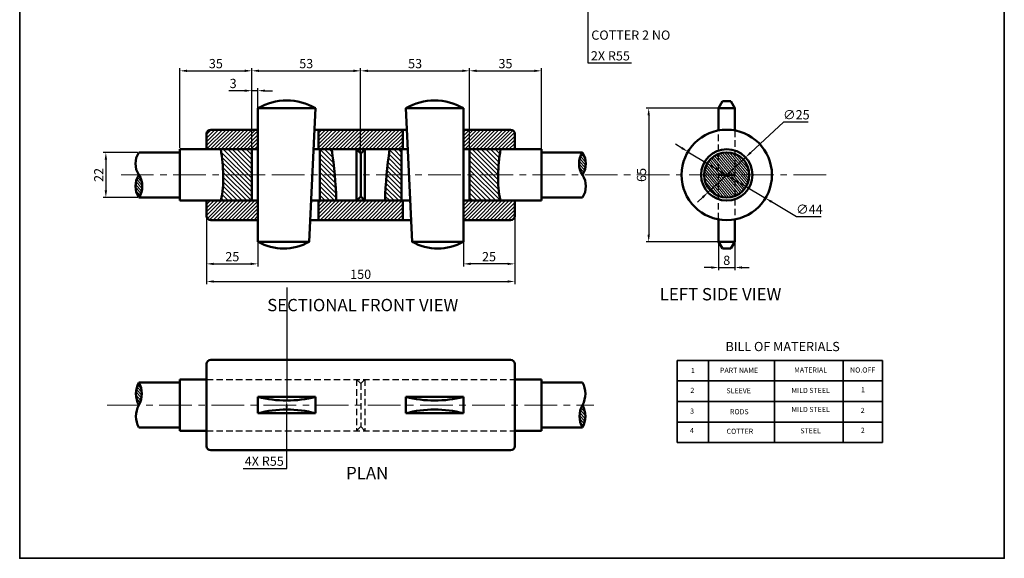
# Model space of a CAD drawing. Units: millimetres. Extents: x -431 to 49, y 153 to 670.
# Tile 1 of 2: x -431 to 49, y 153 to 415. Entities that reach past the tile are written whole.
import ezdxf

# ---------------------------------------------------------------- set-up
doc = ezdxf.new("R2010")
doc.units = ezdxf.units.MM
doc.header["$LTSCALE"] = 0.5
doc.linetypes.add('CENTER', pattern=[50.8, 31.75, -6.35, 6.35, -6.35])
doc.linetypes.add('HIDDEN', pattern=[9.525, 6.35, -3.175])
for name, color, linetype, lineweight in [('M-CNTR', 1, 'CENTER', 18), ('M-DIMS', 2, 'Continuous', 25), ('M-HATC', 8, 'Continuous', 18), ('M-HIDN', 6, 'HIDDEN', 25), ('M-OUTL', 7, 'Continuous', 50), ('M-TEXT', 3, 'Continuous', 25), ('M-TTLB', 7, 'Continuous', 35)]:
    doc.layers.add(name, color=color, linetype=linetype, lineweight=lineweight)
doc.styles.get("Standard").update_dxf_attribs({"font": 'arial.ttf'})
doc.dimstyles.new('ISO-25', dxfattribs={"dimtxt": 4.5, "dimasz": 3.5, "dimexe": 1.25, "dimexo": 0.625, "dimtad": 1, "dimtoh": 1, "dimdec": 0, "dimtxsty": 'Standard', "dimcen": 2.5, "dimadec": 0, "dimazin": 0, "dimtfac": 1, "dimtdec": 0, "dimtmove": 0, "dimatfit": 3, "dimfxl": 1, "dimarcsym": 0})

# ---------------------------------------------------------------- blocks, each defined once
blk = doc.blocks.new('*D14')
at = {"layer": 'Defpoints', "color": 0, "transparency": 16777216}
for p in [(-372.61, 350.31), (-388.68, 328.31), (-372.61, 328.31)]:
    blk.add_point(p, dxfattribs=at)
at = {"layer": 'M-DIMS', "color": 0, "lineweight": -2, "transparency": 16777216}
for p, q in [((-373.23, 350.31), (-389.93, 350.31)), ((-388.68, 346.81), (-388.68, 331.81)), ((-373.23, 328.31), (-389.93, 328.31))]:
    blk.add_line(p, q, dxfattribs=at)
at = {"layer": 'M-DIMS', "color": 0, "transparency": 16777216}
for points in [[(-389.26, 346.81), (-388.1, 346.81), (-388.68, 350.31)], [(-389.26, 331.81), (-388.1, 331.81), (-388.68, 328.31)]]:
    blk.add_solid(points, dxfattribs=at)
at = {"layer": 'M-DIMS', "color": 0, "transparency": 16777216, "insert": (-391.56, 339.31), "char_height": 4.5, "attachment_point": 5, "rotation": 90}
blk.add_mtext('22', dxfattribs=at)
blk = doc.blocks.new('*D15')
at = {"layer": 'Defpoints', "color": 0, "transparency": 16777216}
for p in [(-317.61, 389.99), (-352.61, 351.81), (-317.61, 351.81)]:
    blk.add_point(p, dxfattribs=at)
at = {"layer": 'M-DIMS', "color": 0, "lineweight": -2, "transparency": 16777216}
for p, q in [((-352.61, 352.44), (-352.61, 391.24)), ((-349.11, 389.99), (-321.11, 389.99)), ((-317.61, 352.44), (-317.61, 391.24))]:
    blk.add_line(p, q, dxfattribs=at)
at = {"layer": 'M-DIMS', "color": 0, "transparency": 16777216}
for points in [[(-349.11, 390.58), (-349.11, 389.41), (-352.61, 389.99)], [(-321.11, 390.58), (-321.11, 389.41), (-317.61, 389.99)]]:
    blk.add_solid(points, dxfattribs=at)
at = {"layer": 'M-DIMS', "color": 0, "transparency": 16777216, "insert": (-335.11, 392.92), "char_height": 4.5, "attachment_point": 5}
blk.add_mtext('35', dxfattribs=at)
blk = doc.blocks.new('*D16')
at = {"layer": 'Defpoints', "color": 0, "transparency": 16777216}
for p in [(-317.61, 380.32), (-317.61, 351.81), (-314.61, 351.81)]:
    blk.add_point(p, dxfattribs=at)
at = {"layer": 'M-DIMS', "color": 0, "lineweight": -2, "transparency": 16777216}
for p, q in [((-321.11, 380.32), (-328.81, 380.32)), ((-317.61, 352.44), (-317.61, 381.57)), ((-314.61, 380.32), (-317.61, 380.32)), ((-314.61, 352.44), (-314.61, 381.57)), ((-311.11, 380.32), (-307.61, 380.32))]:
    blk.add_line(p, q, dxfattribs=at)
at = {"layer": 'M-DIMS', "color": 0, "transparency": 16777216}
for points in [[(-321.11, 380.9), (-321.11, 379.74), (-317.61, 380.32)], [(-311.11, 380.9), (-311.11, 379.74), (-314.61, 380.32)]]:
    blk.add_solid(points, dxfattribs=at)
at = {"layer": 'M-DIMS', "color": 0, "transparency": 16777216, "insert": (-326.71, 383.25), "char_height": 4.5, "attachment_point": 5}
blk.add_mtext('3', dxfattribs=at)
blk = doc.blocks.new('*D17')
at = {"layer": 'Defpoints', "color": 0, "transparency": 16777216}
for p in [(-264.61, 389.99), (-317.61, 339.31), (-264.61, 339.31)]:
    blk.add_point(p, dxfattribs=at)
at = {"layer": 'M-DIMS', "color": 0, "lineweight": -2, "transparency": 16777216}
for p, q in [((-317.61, 339.94), (-317.61, 391.24)), ((-314.11, 389.99), (-268.11, 389.99)), ((-264.61, 339.94), (-264.61, 391.24))]:
    blk.add_line(p, q, dxfattribs=at)
at = {"layer": 'M-DIMS', "color": 0, "transparency": 16777216}
for points in [[(-314.11, 390.58), (-314.11, 389.41), (-317.61, 389.99)], [(-268.11, 390.58), (-268.11, 389.41), (-264.61, 389.99)]]:
    blk.add_solid(points, dxfattribs=at)
at = {"layer": 'M-DIMS', "color": 0, "transparency": 16777216, "insert": (-291.11, 392.92), "char_height": 4.5, "attachment_point": 5}
blk.add_mtext('53', dxfattribs=at)
blk = doc.blocks.new('*D18')
at = {"layer": 'Defpoints', "color": 0, "transparency": 16777216}
for p in [(-211.61, 389.99), (-264.61, 339.31), (-211.61, 339.31)]:
    blk.add_point(p, dxfattribs=at)
at = {"layer": 'M-DIMS', "color": 0, "lineweight": -2, "transparency": 16777216}
for p, q in [((-264.61, 339.94), (-264.61, 391.24)), ((-261.11, 389.99), (-215.11, 389.99)), ((-211.61, 339.94), (-211.61, 391.24))]:
    blk.add_line(p, q, dxfattribs=at)
at = {"layer": 'M-DIMS', "color": 0, "transparency": 16777216}
for points in [[(-261.11, 390.58), (-261.11, 389.41), (-264.61, 389.99)], [(-215.11, 390.58), (-215.11, 389.41), (-211.61, 389.99)]]:
    blk.add_solid(points, dxfattribs=at)
at = {"layer": 'M-DIMS', "color": 0, "transparency": 16777216, "insert": (-238.11, 392.92), "char_height": 4.5, "attachment_point": 5}
blk.add_mtext('53', dxfattribs=at)
blk = doc.blocks.new('*D19')
at = {"layer": 'Defpoints', "color": 0, "transparency": 16777216}
for p in [(-176.61, 389.99), (-211.61, 339.31), (-176.61, 339.31)]:
    blk.add_point(p, dxfattribs=at)
at = {"layer": 'M-DIMS', "color": 0, "lineweight": -2, "transparency": 16777216}
for p, q in [((-211.61, 339.94), (-211.61, 391.24)), ((-208.11, 389.99), (-180.11, 389.99)), ((-176.61, 339.94), (-176.61, 391.24))]:
    blk.add_line(p, q, dxfattribs=at)
at = {"layer": 'M-DIMS', "color": 0, "transparency": 16777216}
for points in [[(-208.11, 390.58), (-208.11, 389.41), (-211.61, 389.99)], [(-180.11, 390.58), (-180.11, 389.41), (-176.61, 389.99)]]:
    blk.add_solid(points, dxfattribs=at)
at = {"layer": 'M-DIMS', "color": 0, "transparency": 16777216, "insert": (-194.11, 392.92), "char_height": 4.5, "attachment_point": 5}
blk.add_mtext('35', dxfattribs=at)
blk = doc.blocks.new('*D20')
at = {"layer": 'Defpoints', "color": 0, "transparency": 16777216}
for p in [(-189.61, 326.81), (-339.61, 319.31), (-189.61, 287.45)]:
    blk.add_point(p, dxfattribs=at)
at = {"layer": 'M-DIMS', "color": 0, "lineweight": -2, "transparency": 16777216}
for p, q in [((-189.61, 326.19), (-189.61, 286.2)), ((-339.61, 318.69), (-339.61, 286.2)), ((-336.11, 287.45), (-193.11, 287.45))]:
    blk.add_line(p, q, dxfattribs=at)
at = {"layer": 'M-DIMS', "color": 0, "transparency": 16777216}
for points in [[(-336.11, 288.03), (-336.11, 286.87), (-339.61, 287.45)], [(-193.11, 288.03), (-193.11, 286.87), (-189.61, 287.45)]]:
    blk.add_solid(points, dxfattribs=at)
at = {"layer": 'M-DIMS', "color": 0, "transparency": 16777216, "insert": (-264.61, 290.37), "char_height": 4.5, "attachment_point": 5}
blk.add_mtext('150', dxfattribs=at)
blk = doc.blocks.new('*D21')
at = {"layer": 'Defpoints', "color": 0, "transparency": 16777216}
for p in [(-339.61, 321.31), (-314.61, 321.31), (-314.61, 296.03)]:
    blk.add_point(p, dxfattribs=at)
at = {"layer": 'M-DIMS', "color": 0, "lineweight": -2, "transparency": 16777216}
for p, q in [((-339.61, 320.69), (-339.61, 294.78)), ((-314.61, 320.69), (-314.61, 294.78)), ((-336.11, 296.03), (-318.11, 296.03))]:
    blk.add_line(p, q, dxfattribs=at)
at = {"layer": 'M-DIMS', "color": 0, "transparency": 16777216}
for points in [[(-336.11, 296.61), (-336.11, 295.45), (-339.61, 296.03)], [(-318.11, 296.61), (-318.11, 295.45), (-314.61, 296.03)]]:
    blk.add_solid(points, dxfattribs=at)
at = {"layer": 'M-DIMS', "color": 0, "transparency": 16777216, "insert": (-327.11, 298.95), "char_height": 4.5, "attachment_point": 5}
blk.add_mtext('25', dxfattribs=at)
blk = doc.blocks.new('*D22')
at = {"layer": 'Defpoints', "color": 0, "transparency": 16777216}
for p in [(-214.61, 323.06), (-189.61, 323.06), (-214.61, 296.03)]:
    blk.add_point(p, dxfattribs=at)
at = {"layer": 'M-DIMS', "color": 0, "lineweight": -2, "transparency": 16777216}
for p, q in [((-214.61, 322.44), (-214.61, 294.78)), ((-189.61, 322.44), (-189.61, 294.78)), ((-193.11, 296.03), (-211.11, 296.03))]:
    blk.add_line(p, q, dxfattribs=at)
at = {"layer": 'M-DIMS', "color": 0, "transparency": 16777216}
for points in [[(-211.11, 296.61), (-211.11, 295.45), (-214.61, 296.03)], [(-193.11, 296.61), (-193.11, 295.45), (-189.61, 296.03)]]:
    blk.add_solid(points, dxfattribs=at)
at = {"layer": 'M-DIMS', "color": 0, "transparency": 16777216, "insert": (-202.11, 298.95), "char_height": 4.5, "attachment_point": 5}
blk.add_mtext('25', dxfattribs=at)
blk = doc.blocks.new('*D23')
at = {"layer": 'Defpoints', "color": 0, "transparency": 16777216}
for p in [(-105.24, 350.62), (-67.5, 328.01)]:
    blk.add_point(p, dxfattribs=at)
at = {"layer": 'M-DIMS', "color": 0, "lineweight": -2, "transparency": 16777216}
for p, q in [((-108.24, 352.42), (-111.24, 354.22)), ((-105.24, 350.62), (-67.5, 328.01)), ((-52.4, 318.96), (-64.49, 326.21)), ((-40.45, 318.96), (-52.4, 318.96))]:
    blk.add_line(p, q, dxfattribs=at)
at = {"layer": 'M-DIMS', "color": 0, "transparency": 16777216}
for points in [[(-107.94, 352.92), (-108.54, 351.92), (-105.24, 350.62)], [(-64.19, 326.71), (-64.79, 325.71), (-67.5, 328.01)]]:
    blk.add_solid(points, dxfattribs=at)
at = {"layer": 'M-DIMS', "color": 0, "transparency": 16777216, "insert": (-46.12, 322.01), "char_height": 4.5, "attachment_point": 5}
blk.add_mtext('∅44', dxfattribs=at)
blk = doc.blocks.new('*D24')
at = {"layer": 'Defpoints', "color": 0, "transparency": 16777216}
for p in [(-77.22, 347.83), (-95.52, 330.8)]:
    blk.add_point(p, dxfattribs=at)
at = {"layer": 'M-DIMS', "color": 0, "lineweight": -2, "transparency": 16777216}
for p, q in [((-58.78, 364.97), (-74.65, 350.21)), ((-46.78, 364.97), (-58.78, 364.97)), ((-95.52, 330.8), (-77.22, 347.83)), ((-98.08, 328.42), (-100.65, 326.03))]:
    blk.add_line(p, q, dxfattribs=at)
at = {"layer": 'M-DIMS', "color": 0, "transparency": 16777216}
for points in [[(-75.05, 350.64), (-74.26, 349.78), (-77.22, 347.83)], [(-98.48, 328.84), (-97.69, 327.99), (-95.52, 330.8)]]:
    blk.add_solid(points, dxfattribs=at)
at = {"layer": 'M-DIMS', "color": 0, "transparency": 16777216, "insert": (-52.47, 368.02), "char_height": 4.5, "attachment_point": 5}
blk.add_mtext('∅25', dxfattribs=at)
blk = doc.blocks.new('*D25')
at = {"layer": 'Defpoints', "color": 0, "transparency": 16777216}
for p in [(-90.37, 306.81), (-82.37, 306.81), (-82.37, 294.26)]:
    blk.add_point(p, dxfattribs=at)
at = {"layer": 'M-DIMS', "color": 0, "lineweight": -2, "transparency": 16777216}
for p, q in [((-90.37, 306.19), (-90.37, 293.01)), ((-82.37, 306.19), (-82.37, 293.01)), ((-93.87, 294.26), (-97.37, 294.26)), ((-90.37, 294.26), (-82.37, 294.26)), ((-78.87, 294.26), (-75.37, 294.26))]:
    blk.add_line(p, q, dxfattribs=at)
at = {"layer": 'M-DIMS', "color": 0, "transparency": 16777216}
for points in [[(-93.87, 294.84), (-93.87, 293.67), (-90.37, 294.26)], [(-78.87, 294.84), (-78.87, 293.67), (-82.37, 294.26)]]:
    blk.add_solid(points, dxfattribs=at)
at = {"layer": 'M-DIMS', "color": 0, "transparency": 16777216, "insert": (-86.37, 297.18), "char_height": 4.5, "attachment_point": 5}
blk.add_mtext('8', dxfattribs=at)
blk = doc.blocks.new('*D26')
at = {"layer": 'Defpoints', "color": 0, "transparency": 16777216}
for p in [(-86.37, 371.81), (-124.36, 306.81), (-86.37, 306.81)]:
    blk.add_point(p, dxfattribs=at)
at = {"layer": 'M-DIMS', "color": 0, "lineweight": -2, "transparency": 16777216}
for p, q in [((-86.99, 371.81), (-125.61, 371.81)), ((-124.36, 368.31), (-124.36, 310.31)), ((-86.99, 306.81), (-125.61, 306.81))]:
    blk.add_line(p, q, dxfattribs=at)
at = {"layer": 'M-DIMS', "color": 0, "transparency": 16777216}
for points in [[(-124.95, 368.31), (-123.78, 368.31), (-124.36, 371.81)], [(-124.95, 310.31), (-123.78, 310.31), (-124.36, 306.81)]]:
    blk.add_solid(points, dxfattribs=at)
at = {"layer": 'M-DIMS', "color": 0, "transparency": 16777216, "insert": (-127.29, 339.31), "char_height": 4.5, "attachment_point": 5, "rotation": 90}
blk.add_mtext('65', dxfattribs=at)
blk = doc.blocks.new('COTTER-FRONT')
blk.add_lwpolyline([(28, 65), (28, 0), (3, 0), (0, 65)], close=True)
blk.add_arc((14, 40.75), 28, 60, 120)
blk = doc.blocks.new('COTTER-TOP')
for p, q in [((28, 8), (0, 8)), ((0, 8), (0, 0)), ((28, 0), (28, 8)), ((0, 0), (28, 0))]:
    blk.add_line(p, q)
for centre, start, end in [((14, 61.19), 255.2533, 284.7467), ((14, -53.19), 75.2533, 104.7467)]:
    blk.add_arc(centre, 55, start, end)
blk = doc.blocks.new('*D34')
at = {"layer": 'Defpoints', "color": 0, "ltscale": 0.5, "transparency": 16777216}
for p in [(-153.92, 481.78), (-153.91, 426.78)]:
    blk.add_point(p, dxfattribs=at)
at = {"layer": 'M-DIMS', "color": 0, "lineweight": -2, "ltscale": 0.5, "transparency": 16777216}
for p, q in [((-153.92, 481.78), (-153.91, 426.78)), ((-153.91, 393.78), (-153.91, 423.28)), ((-132.76, 393.78), (-153.91, 393.78))]:
    blk.add_line(p, q, dxfattribs=at)
at = {"layer": 'M-DIMS', "color": 0, "ltscale": 0.5, "transparency": 16777216}
blk.add_solid([(-153.33, 423.28), (-154.5, 423.28), (-153.91, 426.78)], dxfattribs=at)
at = {"layer": 'M-DIMS', "color": 0, "ltscale": 0.5, "transparency": 16777216, "insert": (-143.02, 396.71), "char_height": 4.5, "attachment_point": 5}
blk.add_mtext('2X R55', dxfattribs=at)
blk = doc.blocks.new('*D35')
at = {"layer": 'Defpoints', "color": 0, "ltscale": 0.5, "transparency": 16777216}
for p in [(-300.61, 284.5), (-300.61, 229.5)]:
    blk.add_point(p, dxfattribs=at)
at = {"layer": 'M-DIMS', "color": 0, "lineweight": -2, "ltscale": 0.5, "transparency": 16777216}
for p, q in [((-300.61, 284.5), (-300.61, 229.5)), ((-300.61, 196.5), (-300.61, 226)), ((-321.87, 196.5), (-300.61, 196.5))]:
    blk.add_line(p, q, dxfattribs=at)
at = {"layer": 'M-DIMS', "color": 0, "ltscale": 0.5, "transparency": 16777216}
blk.add_solid([(-301.19, 226), (-300.03, 226), (-300.61, 229.5)], dxfattribs=at)
at = {"layer": 'M-DIMS', "color": 0, "ltscale": 0.5, "transparency": 16777216, "insert": (-311.55, 199.41), "char_height": 4.5, "attachment_point": 5}
blk.add_mtext('4X R55', dxfattribs=at)

msp = doc.modelspace()

# ---------------------------------------------------------------- hatches: boundary and pattern name
at = {"layer": 'M-HATC'}
h = msp.add_hatch(dxfattribs=at)
h.set_pattern_fill('ANSI31', color=256, scale=0.4)
h.paths.add_polyline_path([(-314.609, 361.3128), (-337.609, 361.3128, 0.41421356), (-339.609, 359.3128), (-339.609, 351.8128), (-314.609, 351.8128)])
h.paths.add_polyline_path([(-244.1244, 361.3128), (-285.0936, 361.3128), (-285.0936, 351.8128), (-244.1244, 351.8128)])
h.paths.add_polyline_path([(-189.609, 359.3128, 0.41421356), (-191.609, 361.3128), (-214.609, 361.3128), (-214.609, 351.8128), (-189.609, 351.8128)])
h.paths.add_polyline_path([(-189.609, 326.8128), (-214.609, 326.8128), (-214.609, 317.3128), (-191.609, 317.3128, 0.41421356), (-189.609, 319.3128)])
h.paths.add_polyline_path([(-244.1244, 326.8128), (-285.0936, 326.8128), (-285.0936, 317.3128), (-244.1244, 317.3128)])
h.paths.add_polyline_path([(-314.609, 326.8128), (-339.609, 326.8128), (-339.609, 319.3128, 0.41421356), (-337.609, 317.3128), (-314.609, 317.3128)])
h = msp.add_hatch(dxfattribs=at)
h.set_pattern_fill('ANSI31', color=256, scale=0.5, angle=90)
edge = h.paths.add_edge_path()
edge.add_line((-317.609, 351.8128), (-332.6455, 351.8128))
edge.add_spline(control_points=[(-332.6455, 351.8128), (-332.1521, 347.6251), (-331.6587, 343.4374), (-331.5237, 339.3128)], knot_values=[0, 0, 0, 0, 12.30275825, 12.30275825, 12.30275825, 12.30275825], degree=3, periodic=0)
edge.add_line((-331.5237, 339.3128), (-317.609, 339.3128))
edge.add_line((-317.609, 339.3128), (-317.609, 351.8128))
edge = h.paths.add_edge_path()
edge.add_line((-317.609, 339.3128), (-331.5237, 339.3128))
edge.add_spline(control_points=[(-331.5237, 339.3128), (-331.3844, 335.0558), (-331.627, 330.8661), (-332.6455, 326.8128)], knot_values=[12.30275825, 12.30275825, 12.30275825, 12.30275825, 25, 25, 25, 25], degree=3, periodic=0)
edge.add_line((-332.6455, 326.8128), (-317.609, 326.8128))
edge.add_line((-317.609, 326.8128), (-317.609, 339.3128))
edge = h.paths.add_edge_path()
edge.add_spline(control_points=[(-277.2476, 339.3128), (-277.6434, 343.4827), (-278.1538, 347.6477), (-278.6643, 351.8128)], knot_values=[0, 0, 0, 0, 12.56066367, 12.56066367, 12.56066367, 12.56066367], degree=3, periodic=0)
edge.add_line((-278.6643, 351.8128), (-284.5321, 351.8128))
edge.add_line((-284.5321, 351.8128), (-284.5321, 339.3128))
edge.add_line((-284.5321, 339.3128), (-277.2476, 339.3128))
edge = h.paths.add_edge_path()
edge.add_spline(control_points=[(-276.5193, 326.8128), (-276.572, 330.9876), (-276.8527, 335.1526), (-277.2476, 339.3128)], knot_values=[12.56066367, 12.56066367, 12.56066367, 12.56066367, 25.09185019, 25.09185019, 25.09185019, 25.09185019], degree=3, periodic=0)
edge.add_line((-277.2476, 339.3128), (-284.5321, 339.3128))
edge.add_line((-284.5321, 339.3128), (-284.5321, 326.8128))
edge.add_line((-284.5321, 326.8128), (-276.5193, 326.8128))
h = msp.add_hatch(dxfattribs=at)
h.set_pattern_fill('ANSI31', color=256, scale=0.5, angle=90)
edge = h.paths.add_edge_path()
edge.add_line((-211.609, 351.8128), (-196.5725, 351.8128))
edge.add_spline(control_points=[(-196.5725, 351.8128), (-197.0659, 347.6251), (-197.5594, 343.4374), (-197.6943, 339.3128)], knot_values=[0, 0, 0, 0, 12.30275825, 12.30275825, 12.30275825, 12.30275825], degree=3, periodic=0)
edge.add_line((-197.6943, 339.3128), (-211.609, 339.3128))
edge.add_line((-211.609, 339.3128), (-211.609, 351.8128))
edge = h.paths.add_edge_path()
edge.add_line((-211.609, 339.3128), (-197.6943, 339.3128))
edge.add_spline(control_points=[(-197.6943, 339.3128), (-197.8336, 335.0558), (-197.591, 330.8661), (-196.5725, 326.8128)], knot_values=[12.30275825, 12.30275825, 12.30275825, 12.30275825, 25, 25, 25, 25], degree=3, periodic=0)
edge.add_line((-196.5725, 326.8128), (-211.609, 326.8128))
edge.add_line((-211.609, 326.8128), (-211.609, 339.3128))
edge = h.paths.add_edge_path()
edge.add_spline(control_points=[(-251.9704, 339.3128), (-251.5746, 343.4827), (-251.0642, 347.6477), (-250.5537, 351.8128)], knot_values=[0, 0, 0, 0, 12.56066367, 12.56066367, 12.56066367, 12.56066367], degree=3, periodic=0)
edge.add_line((-250.5537, 351.8128), (-244.6859, 351.8128))
edge.add_line((-244.6859, 351.8128), (-244.6859, 339.3128))
edge.add_line((-244.6859, 339.3128), (-251.9704, 339.3128))
edge = h.paths.add_edge_path()
edge.add_spline(control_points=[(-252.6987, 326.8128), (-252.646, 330.9876), (-252.3653, 335.1526), (-251.9704, 339.3128)], knot_values=[12.56066367, 12.56066367, 12.56066367, 12.56066367, 25.09185019, 25.09185019, 25.09185019, 25.09185019], degree=3, periodic=0)
edge.add_line((-251.9704, 339.3128), (-244.6859, 339.3128))
edge.add_line((-244.6859, 339.3128), (-244.6859, 326.8128))
edge.add_line((-244.6859, 326.8128), (-252.6987, 326.8128))
h = msp.add_hatch(dxfattribs=at)
h.set_pattern_fill('ANSI31', color=256, scale=0.3, angle=85)
h.set_pattern_definition([(130, (180.36415, 264.273), (-0.7296573, -0.6122552), [])])
h.paths.add_polyline_path([(-156.609, 339.3128, 0.29970063), (-156.609, 350.3128, 0.29970063)])
h = msp.add_hatch(dxfattribs=at)
h.set_pattern_fill('ANSI31', color=256, scale=0.3, angle=85)
h.paths.add_polyline_path([(-90.3682, 349.5597, 0.30896041), (-97.3682, 339.3128), (-90.3682, 339.3128)])
h.paths.add_polyline_path([(-82.3682, 349.5597, 0.18826231), (-90.3682, 349.5597), (-90.3682, 339.3128), (-82.3682, 339.3128)])
h.paths.add_polyline_path([(-82.3682, 339.3128), (-90.3682, 339.3128), (-90.3682, 329.0658, 0.18826231), (-82.3682, 329.0658)])
h.paths.add_polyline_path([(-90.3682, 339.3128), (-97.3682, 339.3128, 0.30896041), (-90.3682, 329.0658)])
h.paths.add_polyline_path([(-82.3682, 349.5597), (-82.3682, 339.3128), (-75.3682, 339.3128, 0.30896041)])
h.paths.add_polyline_path([(-75.3682, 339.3128), (-82.3682, 339.3128), (-82.3682, 329.0658, 0.30896041)])
h = msp.add_hatch(dxfattribs=at)
h.set_pattern_fill('ANSI31', color=256, scale=0.3, angle=85)
h.set_pattern_definition([(130, (-476.5793, 264.273), (-0.729657, -0.612255), [])])
h.paths.add_polyline_path([(-372.609, 339.3128, 0.29970063), (-372.609, 328.3128, 0.29970063)])
h = msp.add_hatch(dxfattribs=at)
h.set_pattern_fill('ANSI31', color=256, scale=0.3, angle=85)
h.paths.add_polyline_path([(-372.609, 238.3094, 0.25704732), (-372.609, 227.3094, 0.25704732)])
h.paths.add_polyline_path([(-156.609, 227.3094, 0.25704732), (-156.609, 216.3094, 0.25704732)])

# ---------------------------------------------------------------- linework, layer by layer
at = {"layer": 'M-CNTR'}
for p, q in [((-314.609, 339.3128), (-383.9378, 339.3128)), ((-38.0264, 339.3128), (-314.609, 339.3128)), ((-388.0686, 227.3094), (-151.045, 227.3094))]:
    msp.add_line(p, q, dxfattribs=at)
at = {"layer": 'M-HIDN'}
for p, q in [((-90.3682, 317.6794), (-90.3682, 360.9461)), ((-82.3682, 360.9461), (-82.3682, 317.6794)), ((-339.609, 239.8094), (-189.609, 239.8094)), ((-266.609, 239.8094), (-264.609, 237.8094)), ((-266.609, 239.8094), (-266.609, 214.8094)), ((-262.609, 239.8094), (-264.609, 237.8094)), ((-262.609, 239.8094), (-262.609, 214.8094)), ((-264.609, 237.8094), (-264.609, 216.8094)), ((-266.609, 214.8094), (-264.609, 216.8094)), ((-262.609, 214.8094), (-264.609, 216.8094)), ((-339.609, 214.8094), (-189.609, 214.8094))]:
    msp.add_line(p, q, dxfattribs=at)
at = {"layer": 'M-OUTL'}
for p, q in [((-88.3682, 375.1621), (-90.3682, 371.8128)), ((-88.3682, 375.1621), (-84.3682, 375.1621)), ((-84.3682, 375.1621), (-82.3682, 371.8128)), ((-90.3682, 371.8128), (-90.3682, 360.9461)), ((-82.3682, 371.8128), (-90.3682, 371.8128)), ((-82.3682, 360.9461), (-82.3682, 371.8128)), ((-314.609, 361.3128), (-337.609, 361.3128)), ((-314.609, 361.3128), (-314.609, 351.8128)), ((-242.1244, 361.3128), (-287.0936, 361.3128)), ((-285.0936, 361.3128), (-285.0936, 351.8128)), ((-242.1244, 361.3128), (-244.1244, 361.3128)), ((-244.1244, 361.3128), (-244.1244, 351.8128)), ((-214.609, 351.8128), (-214.609, 361.3128)), ((-191.609, 361.3128), (-214.609, 361.3128)), ((-339.609, 359.3128), (-339.609, 351.8128)), ((-189.609, 351.8128), (-189.609, 359.3128)), ((-352.609, 350.3128), (-372.609, 350.3128)), ((-352.609, 351.8128), (-314.609, 351.8128)), ((-352.609, 326.8128), (-352.609, 351.8128)), ((-339.609, 351.8128), (-314.609, 351.8128)), ((-317.609, 326.8128), (-317.609, 351.8128)), ((-287.5321, 351.8128), (-266.609, 351.8128)), ((-287.5321, 351.8128), (-241.6859, 351.8128)), ((-284.5321, 351.8128), (-284.5321, 326.8128)), ((-266.609, 351.8128), (-264.609, 349.8128)), ((-266.609, 351.8128), (-266.609, 326.8128)), ((-262.609, 351.8128), (-264.609, 349.8128)), ((-262.609, 351.8128), (-262.609, 326.8128)), ((-241.6859, 351.8128), (-262.609, 351.8128)), ((-244.6859, 351.8128), (-244.6859, 326.8128)), ((-176.609, 351.8128), (-214.609, 351.8128)), ((-214.609, 351.8128), (-189.609, 351.8128)), ((-211.609, 326.8128), (-211.609, 351.8128)), ((-176.609, 326.8128), (-176.609, 351.8128)), ((-176.609, 350.3128), (-156.609, 350.3128)), ((-264.609, 349.8128), (-264.609, 328.8128)), ((-264.609, 349.8128), (-264.609, 328.8128)), ((-82.3682, 339.3128), (-90.3682, 339.3128)), ((-372.609, 328.3128), (-352.609, 328.3128)), ((-314.609, 326.8128), (-352.609, 326.8128)), ((-339.609, 326.8128), (-314.609, 326.8128)), ((-339.609, 326.8128), (-339.609, 319.3128)), ((-314.609, 326.8128), (-314.609, 317.3128)), ((-266.609, 326.8128), (-288.6859, 326.8128)), ((-288.6859, 326.8128), (-240.5321, 326.8128)), ((-285.0936, 326.8128), (-285.0936, 317.3128)), ((-266.609, 326.8128), (-264.609, 328.8128)), ((-262.609, 326.8128), (-264.609, 328.8128)), ((-262.609, 326.8128), (-240.5321, 326.8128)), ((-244.1244, 326.8128), (-244.1244, 317.3128)), ((-214.609, 317.3128), (-214.609, 326.8128)), ((-214.609, 326.8128), (-176.609, 326.8128)), ((-214.609, 326.8128), (-189.609, 326.8128)), ((-189.609, 319.3128), (-189.609, 326.8128)), ((-156.609, 328.3128), (-176.609, 328.3128)), ((-337.609, 317.3128), (-314.609, 317.3128)), ((-289.1244, 317.3128), (-240.0936, 317.3128)), ((-214.609, 317.3128), (-191.609, 317.3128)), ((-90.3682, 317.6794), (-90.3682, 306.8128)), ((-82.3682, 306.8128), (-82.3682, 317.6794)), ((-90.3682, 306.8128), (-82.3682, 306.8128)), ((-88.3682, 303.4634), (-90.3682, 306.8128)), ((-88.3682, 303.4634), (-84.3682, 303.4634)), ((-84.3682, 303.4634), (-82.3682, 306.8128)), ((-191.609, 249.3094), (-337.609, 249.3094)), ((-242.1244, 249.3094), (-244.1244, 249.3094)), ((-339.609, 247.3094), (-339.609, 207.3094)), ((-189.609, 207.3094), (-189.609, 247.3094)), ((-339.609, 239.8094), (-352.609, 239.8094)), ((-352.609, 239.8094), (-352.609, 214.8094)), ((-189.609, 239.8094), (-176.609, 239.8094)), ((-176.609, 239.8094), (-176.609, 214.8094)), ((-352.609, 238.3094), (-372.609, 238.3094)), ((-176.609, 238.3094), (-156.609, 238.3094)), ((-352.609, 216.3094), (-372.609, 216.3094)), ((-176.609, 216.3094), (-156.609, 216.3094)), ((-352.609, 214.8094), (-339.609, 214.8094)), ((-189.609, 214.8094), (-176.609, 214.8094)), ((-337.609, 205.3094), (-191.609, 205.3094))]:
    msp.add_line(p, q, dxfattribs=at)
for radius in [22, 12.5, 11]:
    msp.add_circle((-86.3682, 339.3128), radius, dxfattribs=at)
for centre, radius, start, end in [((-337.609, 359.3128), 2, 90, 180), ((-191.609, 359.3128), 2, 0, 90), ((-364.2574, 344.8128), 10, 146.632987, 213.367013), ((-148.2574, 344.8128), 10, 146.632987, 213.367013), ((-164.9607, 344.8128), 10, 326.632987, 33.367013), ((-364.2574, 333.8128), 10, 146.632987, 213.367013), ((-380.9607, 333.8128), 10, 326.632987, 33.367013), ((-164.9607, 333.8128), 10, 326.632987, 33.367013), ((-337.609, 319.3128), 2, 180, 270), ((-191.609, 319.3128), 2, 270, 0), ((-302.109, 328.4634), 25, 240, 300), ((-227.109, 328.4634), 25, 240, 300), ((-337.609, 247.3094), 2, 90, 180), ((-191.609, 247.3094), 2, 0, 90), ((-362.6175, 232.8094), 11.4053, 151.168723, 208.831277), ((-382.6005, 232.8094), 11.4053, 331.168723, 28.831277), ((-166.6005, 232.8094), 11.4053, 331.168723, 28.831277), ((-362.6175, 221.8094), 11.4053, 151.168723, 208.831277), ((-146.6175, 221.8094), 11.4053, 151.168723, 208.831277), ((-166.6005, 221.8094), 11.4053, 331.168723, 28.831277), ((-337.609, 207.3094), 2, 180, 270), ((-191.609, 207.3094), 2, 270, 0)]:
    msp.add_arc(centre, radius, start, end, dxfattribs=at)
for points in [[(-332.6455, 351.8128), (-331.6428, 343.3031), (-330.6402, 334.7935), (-332.6455, 326.8128)], [(-278.6643, 351.8128), (-277.6446, 343.4925), (-276.6249, 335.1722), (-276.5193, 326.8128)], [(-250.5537, 351.8128), (-251.5734, 343.4925), (-252.5931, 335.1722), (-252.6987, 326.8128)], [(-196.5725, 351.8128), (-197.5752, 343.3031), (-198.5778, 334.7935), (-196.5725, 326.8128)]]:
    msp.add_open_spline(points, degree=3, dxfattribs=at)
at = {"layer": 'M-TTLB', "ltscale": 0.5}
for p, q in [((-110.4778, 249.0446), (-10.4778, 249.0446)), ((-110.4778, 249.0446), (-110.4778, 239.0446)), ((-110.4778, 209.0446), (-110.4778, 249.0446)), ((-95.2897, 249.0446), (-95.2897, 209.0446)), ((-63.0803, 249.0446), (-63.0803, 209.0446)), ((-29.6641, 249.0446), (-29.6641, 209.0446)), ((-10.4778, 249.0446), (-10.4778, 209.0446)), ((-110.4778, 239.0446), (-10.4778, 239.0446)), ((-110.4778, 229.0446), (-10.4778, 229.0446)), ((-110.4778, 219.0446), (-10.4778, 219.0446)), ((-110.4778, 209.0446), (-10.4778, 209.0446))]:
    msp.add_line(p, q, dxfattribs=at)
msp.add_lwpolyline([(-430.6355, 670.1955), (48.7912, 670.1955), (48.7912, 152.7108), (-430.6355, 152.7108)], close=True, dxfattribs=at)

# ---------------------------------------------------------------- block references
at = {"layer": 'M-OUTL', "extrusion": (0, 0, -1), "zscale": -1}
msp.add_blockref('COTTER-FRONT', (286.6094, 306.8131), dxfattribs=at)
at = {"layer": 'M-OUTL'}
for name, p in [('COTTER-FRONT', (-242.6086, 306.8131)), ('COTTER-TOP', (-314.6086, 223.3098)), ('COTTER-TOP', (-242.6086, 223.3098))]:
    msp.add_blockref(name, p, dxfattribs=at)

# ---------------------------------------------------------------- texts
at = {"layer": 'M-TEXT', "attachment_point": 1}
for s, width, insert, char_height in [('\\pxqc;COTTER 2 NO', 77.714637, (-171.9292, 409.6228), 4.5), ('\\pxqc;LEFT SIDE VIEW', 108.244216, (-143.4994, 284.2609), 6), ('\\pxqc;SECTIONAL FRONT VIEW', 108.244216, (-317.7204, 278.9737), 6), ('\\pxqc;PLAN', 20.816312, (-271.8366, 197.2278), 6)]:
    msp.add_mtext_dynamic_manual_height_columns(s, width=width, gutter_width=12.5, heights=[0], dxfattribs=dict(at, insert=insert, char_height=char_height))
at = {"layer": 'M-TEXT', "insert": (-113.2668, 258.0382), "char_height": 4.5, "width": 108.244216, "attachment_point": 1}
msp.add_mtext('\\pxqc;BILL OF MATERIALS', dxfattribs=at)
at = {"layer": 'M-TEXT', "ltscale": 0.5, "char_height": 2.5, "attachment_point": 1}
for s, width, insert in [('\\pxqc;1', 10.661826, (-108.1985, 245.3917)), ('\\pxqc;PART NAME', 20.703013, (-90.7262, 245.4623)), ('\\pxqc;MATERIAL', 20.703013, (-55.8839, 245.6305)), ('\\pxqc;NO.OFF', 10.661826, (-25.524, 245.6108)), ('\\pxqc;2', 10.661826, (-108.4694, 235.7147)), ('\\pxqc;SLEEVE', 10.661826, (-85.8697, 235.5015)), ('\\pxqc;MILD STEEL', 20.703013, (-55.8839, 235.6629)), ('\\pxqc;1', 10.661826, (-25.3392, 236.0236)), ('\\pxqc;3', 10.661826, (-108.5921, 225.5983)), ('\\pxqc;RODS', 10.661826, (-85.5754, 225.3088)), ('\\pxqc;MILD STEEL', 20.703013, (-55.8839, 226.3995)), ('\\pxqc;2', 10.661826, (-25.5344, 225.9417)), ('\\pxqc;4', 10.661826, (-108.6676, 216.1502)), ('\\pxqc;COTTER', 10.661826, (-85.2811, 215.8022)), ('\\pxqc;STEEL', 20.703013, (-55.8839, 216.0194)), ('\\pxqc;2', 10.661826, (-25.4356, 216.2705))]:
    msp.add_mtext_dynamic_manual_height_columns(s, width=width, gutter_width=12.5, heights=[0], dxfattribs=dict(at, insert=insert))

# ---------------------------------------------------------------- dimensions: what is measured, and where the dimension line sits
at = {"layer": 'M-DIMS', "ltscale": 0.5}
for center, mpoint, text, picture, middle in [((-153.9154, 481.785), (-153.915, 426.785), '2X <>', '*D34', (-143.0236, 393.785)), ((-300.609, 284.4978), (-300.609, 229.4978), '4X <>', '*D35', (-311.5524, 196.4978))]:
    dim = msp.add_radius_dim(center=center, mpoint=mpoint, text=text, dimstyle='ISO-25', override={"dimdec": 0, "dimlfac": 1, "dimrnd": 0, "dimzin": 0, "dimdsep": 46, "dimlunit": 2}, dxfattribs=at)
    dim.commit()
    dim.dimension.update_dxf_attribs({"geometry": picture, "text_midpoint": middle, "dimtype": 164})
at = {"layer": 'M-DIMS'}
for base, p1, p2, picture, middle in [((-317.609, 389.9937), (-352.609, 351.8128), (-317.609, 351.8128), '*D15', (-335.109, 392.9178)), ((-264.609, 389.9937), (-317.609, 339.3128), (-264.609, 339.3128), '*D17', (-291.109, 392.9178)), ((-211.609, 389.9937), (-264.609, 339.3128), (-211.609, 339.3128), '*D18', (-238.109, 392.9178)), ((-176.609, 389.9937), (-211.609, 339.3128), (-176.609, 339.3128), '*D19', (-194.109, 392.9178)), ((-317.609, 380.3212), (-314.609, 351.8128), (-317.609, 351.8128), '*D16', (-326.7074, 383.2453)), ((-189.609, 287.4486), (-339.609, 319.3128), (-189.609, 326.8128), '*D20', (-264.609, 290.3712)), ((-314.609, 296.0284), (-339.609, 321.3128), (-314.609, 321.3128), '*D21', (-327.109, 298.951)), ((-214.609, 296.0284), (-189.609, 323.0628), (-214.609, 323.0628), '*D22', (-202.109, 298.951)), ((-82.3682, 294.256), (-90.3682, 306.8128), (-82.3682, 306.8128), '*D25', (-86.3682, 297.1786))]:
    dim = msp.add_linear_dim(base=base, p1=p1, p2=p2, dimstyle='ISO-25', override={"dimclrd": 0, "dimclre": 0, "dimclrt": 0}, dxfattribs=at)
    dim.commit()
    dim.dimension.update_dxf_attribs({"geometry": picture, "text_midpoint": middle})
for base, p1, p2, picture, middle in [((-124.3643, 306.8128), (-86.3682, 371.8128), (-86.3682, 306.8128), '*D26', (-127.2868, 339.3128)), ((-388.6791, 328.3128), (-372.609, 350.3128), (-372.609, 328.3128), '*D14', (-391.5633, 339.3128))]:
    dim = msp.add_linear_dim(base=base, p1=p1, p2=p2, angle=90, dimstyle='ISO-25', override={"dimclrd": 0, "dimclre": 0, "dimclrt": 0}, dxfattribs=at)
    dim.commit()
    dim.dimension.update_dxf_attribs({"geometry": picture, "text_midpoint": middle})
for p1, p2, picture, middle in [((-95.5206, 330.799), (-77.2159, 347.8265), '*D24', (-52.4714, 364.9721)), ((-105.2402, 350.6198), (-67.4962, 328.0057), '*D23', (-46.1167, 318.9631))]:
    dim = msp.add_diameter_dim_2p(p1=p1, p2=p2, dimstyle='ISO-25', override={"dimclrd": 0, "dimclre": 0, "dimclrt": 0}, dxfattribs=at)
    dim.commit()
    dim.dimension.update_dxf_attribs({"geometry": picture, "text_midpoint": middle, "dimtype": 163})

doc.saveas('drawing.dxf')
